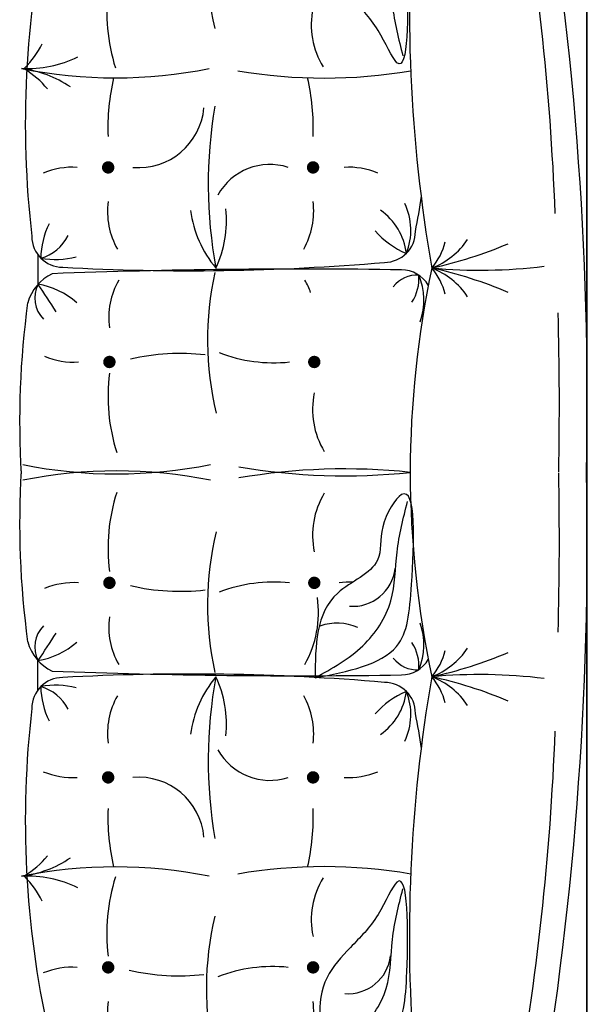
# Model space of a CAD drawing. Units: inches. Extents: x 844 to 2234, y 346 to 1084.
# Tile 40 of 93: x 1269 to 1284, y 682 to 708. Entities that reach past the tile are written whole.
import ezdxf

# ---------------------------------------------------------------- set-up
doc = ezdxf.new("R2010")
doc.units = ezdxf.units.IN
doc.header["$MEASUREMENT"] = 0
doc.layers.add('A-WALL', color=7, linetype='Continuous', lineweight=35)
doc.layers.add('furniture', color=8, linetype='Continuous', lineweight=18)
doc.layers.add('RA-AP-01$0$FURN', color=3, linetype='Continuous')
doc.layers.add('RA-AP-01$0$WOOD', color=64, linetype='Continuous')

# ---------------------------------------------------------------- blocks, each defined once
blk = doc.blocks.new('A$C7EE91E48')
at = {"layer": 'RA-AP-01$0$FURN'}
for p, q in [((8.4752, -8.8836), (8.5044, -8.8836)), ((8.5044, -8.8836), (8.5227, -8.8836)), ((9.1476, -8.8836), (9.1292, -8.8836)), ((9.1768, -8.8836), (9.1476, -8.8836))]:
    blk.add_line(p, q, dxfattribs=at)
at = {"layer": 'RA-AP-01$0$FURN', "const_width": 0.01}
for points in [[(8.0279, -9.0019, -1), (8.0279, -8.9919, -1)], [(8.3342, -9.0019, 1), (8.3342, -8.9919, 1)], [(8.6479, -9.0039, -1), (8.6479, -8.9939, -1)], [(9.004, -9.0039, 1), (9.004, -8.9939, 1)], [(9.3177, -9.0019, -1), (9.3177, -8.9919, -1)], [(8.0279, -9.3223, 1), (8.0279, -9.3323, 1)], [(8.3342, -9.3223, -1), (8.3342, -9.3323, -1)], [(9.3177, -9.3223, 1), (9.3177, -9.3323, 1)], [(8.6479, -9.3243, 1), (8.6479, -9.3343, 1)], [(9.004, -9.3243, -1), (9.004, -9.3343, -1)]]:
    blk.add_lwpolyline(points, format="xyb", close=True, dxfattribs=at)
at = {"layer": 'RA-AP-01$0$FURN'}
for centre, radius, start, end in [((7.9834, -8.8653), 0.1916, 334.4169, 2.4147), ((7.4244, -9.0082), 0.7655, 348.5826, 11.3727), ((8.3595, -8.8326), 0.1864, 187.6182, 213.7074), ((8.744, -10.2748), 1.4207, 86.5948, 97.7424), ((8.9079, -10.2748), 1.4207, 82.2576, 93.4052), ((9.2924, -8.8326), 0.1864, 326.2926, 352.3818), ((10.2276, -9.0082), 0.7655, 168.6273, 191.4174), ((9.6686, -8.8653), 0.1916, 177.5853, 205.5831), ((8.2641, -10.4424), 1.5791, 83.4116, 102.408), ((8.0633, -8.7497), 0.1579, 296.9155, 314.5948), ((8.3098, -8.7788), 0.1579, 211.9342, 229.6135), ((8.4452, -8.9237), 0.05, 0, 90), ((8.5734, -8.9396), 0.0754, 106.0166, 154.1254), ((8.0629, -9.0102), 0.7655, 348.5826, 11.3727), ((9.589, -9.0102), 0.7655, 168.6273, 191.4174), ((9.0785, -8.9396), 0.0754, 25.8746, 73.9834), ((9.2067, -8.9237), 0.05, 90, 180), ((9.3879, -10.4424), 1.5791, 77.592, 96.5884), ((9.3421, -8.7788), 0.1579, 310.3865, 328.0658), ((9.5886, -8.7497), 0.1579, 225.4052, 243.0845), ((8.4834, -9.0206), 0.1324, 91.1993, 116.1112), ((8.411, -8.8679), 0.0726, 297.3225, 343.6441), ((8.3504, -8.912), 0.1324, 345.3922, 10.3041), ((8.5446, -8.9264), 0.0479, 44.5975, 117.1929), ((8.6431, -8.8646), 0.1219, 188.9538, 221.9624), ((9.1542, -7.9707), 1.1102, 235.3335, 238.0671), ((9.1073, -8.9264), 0.0479, 62.8071, 135.4025), ((8.4977, -7.9707), 1.1102, 301.9329, 304.6665), ((9.0089, -8.8646), 0.1219, 318.0376, 351.0462), ((9.3016, -8.912), 0.1324, 169.6959, 194.6078), ((9.1686, -9.0206), 0.1324, 63.8888, 88.8007), ((9.241, -8.8679), 0.0726, 196.3559, 242.6775), ((7.9069, -8.939), 0.1213, 356.2685, 22.6624), ((8.4553, -8.939), 0.1213, 157.3376, 183.7315), ((8.5269, -8.941), 0.1213, 356.2685, 22.6624), ((9.1251, -8.941), 0.1213, 157.3376, 183.7315), ((9.1967, -8.939), 0.1213, 356.2685, 22.6624), ((19.2274, -9.306), 10.7293, 177.86728, 180.87576), ((-1.5755, -9.306), 10.7293, 359.12424, 2.13272), ((4.8029, -9.1271), 3.698, 355.1082, 3.1536), ((12.8491, -9.1271), 3.698, 176.8464, 184.8918), ((7.9567, -9.1172), 0.1214, 82.3083, 119.8581), ((8.0823, -9.2969), 0.3024, 72.4119, 96.9055), ((8.2692, -9.3452), 0.3487, 87.5342, 103.1608), ((8.4055, -9.1172), 0.1214, 60.1419, 97.6917), ((8.5767, -9.1192), 0.1214, 82.3083, 119.8581), ((8.7023, -9.299), 0.3024, 72.4119, 96.9055), ((8.9496, -9.299), 0.3024, 83.0945, 107.5881), ((9.0753, -9.1192), 0.1214, 60.1419, 97.6917), ((9.2465, -9.1172), 0.1214, 82.3083, 119.8581), ((9.3827, -9.3452), 0.3487, 76.8392, 92.4658), ((9.5696, -9.2969), 0.3024, 83.0945, 107.5881), ((8.3659, -9.111), 0.3517, 166.8325, 186.5875), ((8.9859, -9.113), 0.3517, 166.8325, 186.5875), ((8.666, -9.113), 0.3517, 353.4125, 13.1675), ((8.2285, -9.0458), 0.106, 275.1859, 4.8073), ((9.4234, -9.0458), 0.106, 175.1927, 264.8141), ((8.378, -9.3133), 0.1855, 50.3168, 82.0523), ((9.2739, -9.3133), 0.1855, 97.9477, 129.6832), ((7.9929, -9.6653), 0.5101, 76.6878, 102.3818), ((8.3614, -9.9068), 0.7485, 79.6011, 99.6906), ((8.6129, -9.6673), 0.5101, 76.6878, 102.3818), ((9.0391, -9.6673), 0.5101, 77.6182, 103.3122), ((9.2906, -9.9068), 0.7485, 80.3094, 100.3989), ((9.6591, -9.6653), 0.5101, 77.6182, 103.3122), ((7.785, -9.2618), 0.2442, 354.0076, 21.0983), ((8.4248, -9.2574), 0.0954, 118.8034, 198.2253), ((8.4207, -9.0107), 0.1769, 263.6796, 295.3608), ((8.405, -9.2638), 0.2442, 354.0076, 21.0983), ((9.2469, -9.2638), 0.2442, 158.9017, 185.9924), ((9.2312, -9.0107), 0.1769, 244.6392, 276.3204), ((9.2271, -9.2574), 0.0954, 341.7747, 61.1966), ((7.367, -9.3453), 0.8233, 350.2449, 9.7551), ((7.8327, -9.3782), 0.9989, 353.9343, 9.823), ((9.8193, -9.3782), 0.9989, 170.177, 186.0657), ((10.285, -9.3453), 0.8233, 170.2449, 189.7551), ((7.9567, -9.2069), 0.1214, 240.1419, 277.6917), ((8.2692, -8.9789), 0.3487, 256.8392, 272.4658), ((8.4055, -9.2069), 0.1214, 262.3083, 299.8581), ((8.6002, -9.1634), 0.1726, 240.9024, 278.0073), ((9.0753, -9.209), 0.1214, 289.6086, 299.8581), ((9.2465, -9.2069), 0.1214, 240.1419, 277.6917), ((9.3827, -8.9789), 0.3487, 267.5342, 283.1608), ((8.1048, -9.4539), 0.1295, 58.6204, 102.0099), ((8.7248, -9.456), 0.1295, 58.6204, 102.0099), ((8.9271, -9.456), 0.1295, 77.9901, 121.3796), ((9.5471, -9.4539), 0.1295, 77.9901, 121.3796), ((8.5004, -9.3657), 0.0825, 335.8161, 19.2747), ((8.0543, -9.3837), 0.0689, 175.5384, 263.5805), ((8.4553, -9.3851), 0.1213, 176.2685, 202.6624), ((8.405, -9.3948), 0.2442, 0.7304, 5.9924), ((9.1967, -9.3851), 0.1213, 337.3376, 3.7315), ((8.6789, -9.3912), 0.0689, 175.5384, 263.5805), ((8.3451, -9.5317), 0.1386, 22.9132, 48.7711), ((9.3068, -9.5317), 0.1386, 131.2289, 157.0868), ((8.4847, -9.3794), 0.0991, 214.8912, 263.0774), ((8.4374, -9.4424), 0.05, 270, 0), ((9.2146, -9.4424), 0.05, 180, 270), ((9.1673, -9.3794), 0.0991, 276.9226, 325.1088), ((8.5556, -9.4948), 0.0479, 127.3166, 183.4247), ((9.0963, -9.4948), 0.0479, 356.5753, 52.6834), ((8.4354, -9.3857), 0.0993, 244.3656, 292.0953), ((8.5494, -9.4699), 0.05, 180, 239.8522), ((9.1025, -9.4699), 0.05, 300.1478, 360), ((9.2166, -9.3857), 0.0993, 247.9047, 295.6344), ((8.0772, -11.9348), 2.4522, 80.1542, 94.8039), ((8.1811, -8.1864), 1.3309, 278.6229, 281.1036), ((8.8331, -11.1187), 1.6349, 90.2483, 101.88), ((8.514, -9.4297), 0.0683, 264.7816, 303.327), ((8.8189, -11.1187), 1.6349, 78.12, 89.7517), ((9.1379, -9.4297), 0.0683, 236.673, 275.2184), ((9.5748, -11.9348), 2.4522, 85.1961, 99.8458), ((9.4709, -8.1864), 1.3309, 258.8964, 261.3771), ((8.5483, -9.4017), 0.1042, 247.1307, 289.5172), ((9.1036, -9.4017), 0.1042, 250.4828, 292.8693), ((8.3825, -9.4751), 0.122, 303.7136, 339.041), ((8.4279, -9.4377), 0.1062, 284.3648, 310.2303), ((7.8141, -9.3689), 0.6986, 337.0091, 347.612), ((7.6413, -9.5958), 0.8587, 353.0376, 5.1445), ((8.6105, -9.4751), 0.122, 200.959, 236.2864), ((8.5651, -9.4377), 0.1062, 229.7697, 255.6352), ((9.1788, -9.3689), 0.6986, 192.388, 202.9909), ((9.0415, -9.4751), 0.122, 303.7136, 339.041), ((9.0869, -9.4377), 0.1062, 284.3648, 310.2303), ((8.4731, -9.3689), 0.6986, 337.0091, 347.612), ((10.0107, -9.5958), 0.8587, 174.8555, 186.9624), ((9.2694, -9.4751), 0.122, 200.959, 236.2864), ((9.224, -9.4377), 0.1062, 229.7697, 255.6352), ((9.8378, -9.3689), 0.6986, 192.388, 202.9909), ((8.5724, -5.4361), 4.2848, 259.7801, 267.8084), ((9.0796, -5.4361), 4.2848, 272.1916, 280.2199), ((8.7159, -4.2841), 5.4854, 259.9939, 271.1496), ((8.936, -4.2841), 5.4854, 268.8504, 280.0061), ((8.7159, -4.2841), 5.4404, 268.4485, 271.1496), ((8.936, -4.2841), 5.4404, 268.8504, 271.5515)]:
    blk.add_arc(centre, radius, start, end, dxfattribs=at)
for points, knots in [([(7.8747, -9.3485), (7.9231, -9.3393), (7.9933, -9.326), (8.0638, -9.3901), (8.1031, -9.4315), (8.221, -9.4812), (8.0194, -9.4811), (7.9064, -9.4702), (7.8857, -9.3906), (7.8747, -9.3485)], [0, 0, 0, 0, 0.1367587, 0.1981302, 0.267773, 0.3281195, 0.4737578, 0.5765194, 0.6920332, 0.6920332, 0.6920332, 0.6920332]), ([(8.4947, -9.3305), (8.5098, -9.3579), (8.5387, -9.4102), (8.6151, -9.4603), (8.6994, -9.4595), (8.7521, -9.4728), (8.7791, -9.4797)], [0, 0, 0, 0, 0.0929945, 0.178054, 0.2574251, 0.3407808, 0.3407808, 0.3407808, 0.3407808]), ([(8.4947, -9.3305), (8.547, -9.3311), (8.63, -9.3319), (8.67, -9.4425), (8.7389, -9.4316), (8.8424, -9.4963), (8.6448, -9.4874), (8.5233, -9.4759), (8.5051, -9.3838), (8.4947, -9.3305)], [0, 0, 0, 0, 0.1415752, 0.2249019, 0.2789443, 0.3392908, 0.4849291, 0.5876907, 0.7285367, 0.7285367, 0.7285367, 0.7285367]), ([(9.7773, -9.3485), (9.7288, -9.3393), (9.6586, -9.326), (9.5882, -9.3901), (9.5488, -9.4315), (9.4309, -9.4812), (9.6325, -9.4811), (9.7455, -9.4702), (9.7663, -9.3906), (9.7773, -9.3485)], [0, 0, 0, 0, 0.1367587, 0.1981302, 0.267773, 0.3281195, 0.4737578, 0.5765194, 0.6920332, 0.6920332, 0.6920332, 0.6920332]), ([(7.8747, -9.3485), (7.8896, -9.3663), (7.9228, -9.4056), (7.9899, -9.4532), (8.0749, -9.4519), (8.1275, -9.4653), (8.1544, -9.4722)], [0, 0, 0, 0, 0.0700185, 0.155078, 0.2344492, 0.3178049, 0.3178049, 0.3178049, 0.3178049]), ([(9.7773, -9.3485), (9.7623, -9.3663), (9.7292, -9.4056), (9.662, -9.4532), (9.577, -9.4519), (9.5245, -9.4653), (9.4975, -9.4722)], [0, 0, 0, 0, 0.0700185, 0.155078, 0.2344492, 0.3178049, 0.3178049, 0.3178049, 0.3178049])]:
    blk.add_open_spline(points, degree=3, knots=knots, dxfattribs=at)
blk = doc.blocks.new('A$C5D2F253E')
at = {"layer": 'RA-AP-01$0$WOOD', "xscale": -1, "rotation": 180}
blk.add_blockref('A$C7EE91E48', (-8.833, -7.2888), dxfattribs=at)

msp = doc.modelspace()

# ---------------------------------------------------------------- linework, layer by layer
at = {"layer": 'A-WALL'}
msp.add_line((1283.616, 761.311), (1283.616, 624.311), dxfattribs=at)

# ---------------------------------------------------------------- block references
at = {"layer": 'furniture', "xscale": -15.94108302203742, "yscale": 15.94108302203742, "zscale": 15.94108302203742, "rotation": 270}
msp.add_blockref('A$C5D2F253E', (1244.084, 696.258), dxfattribs=at)

doc.saveas('drawing.dxf')
